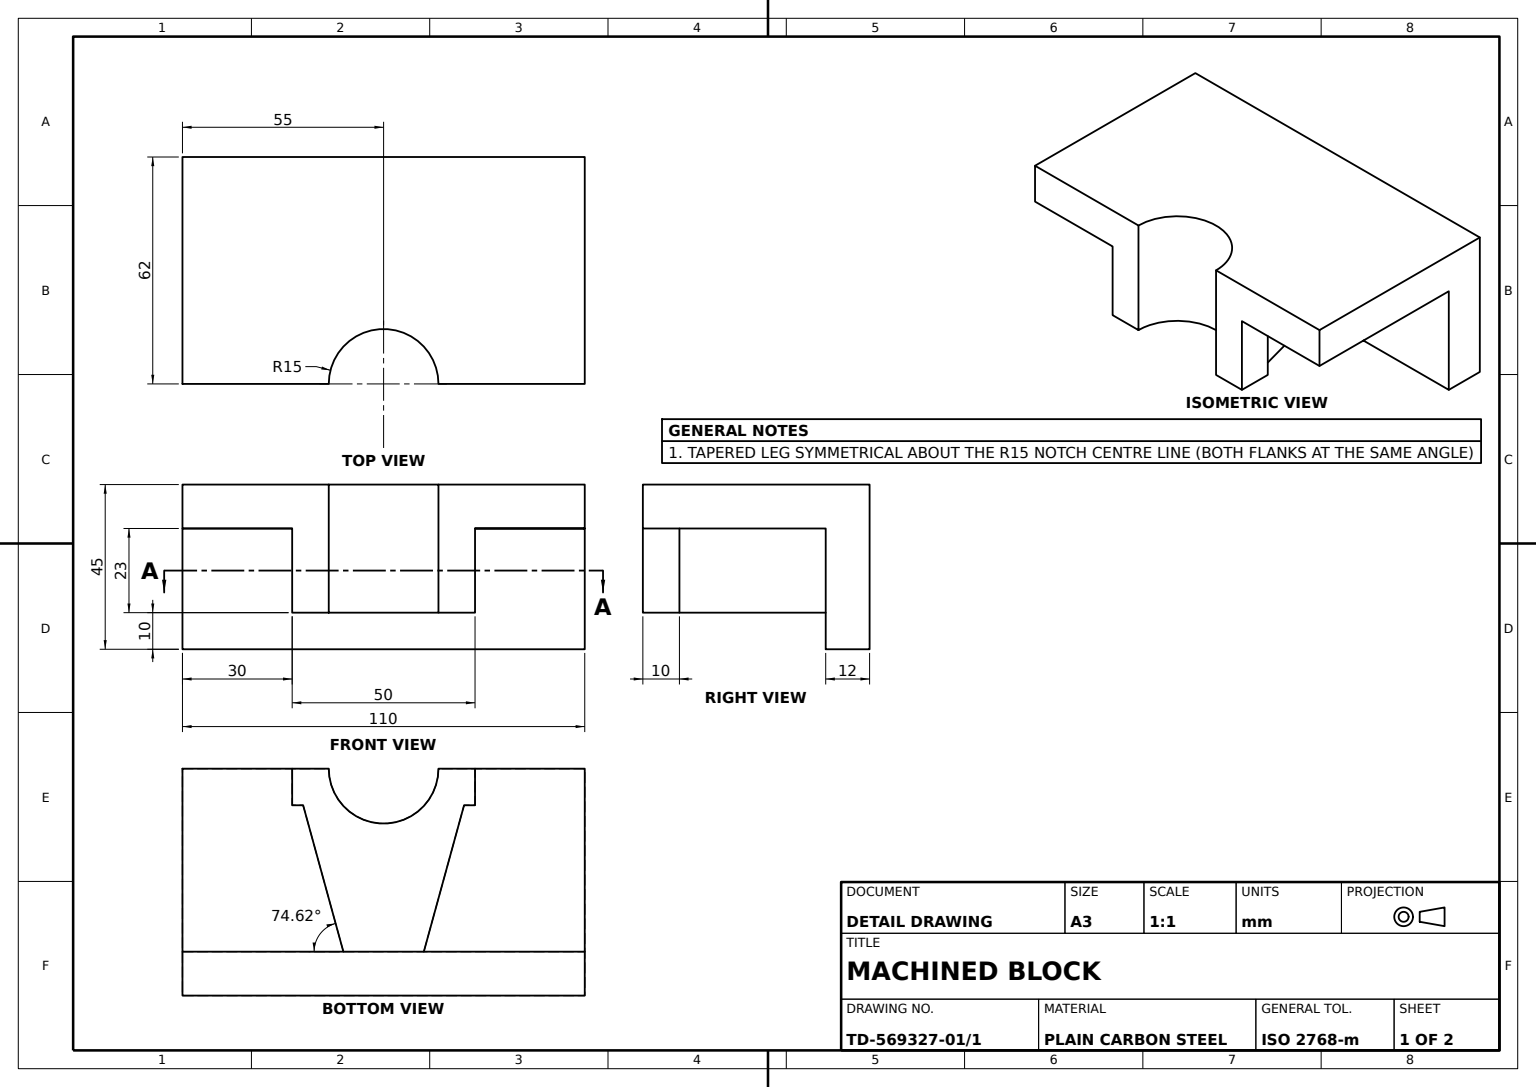
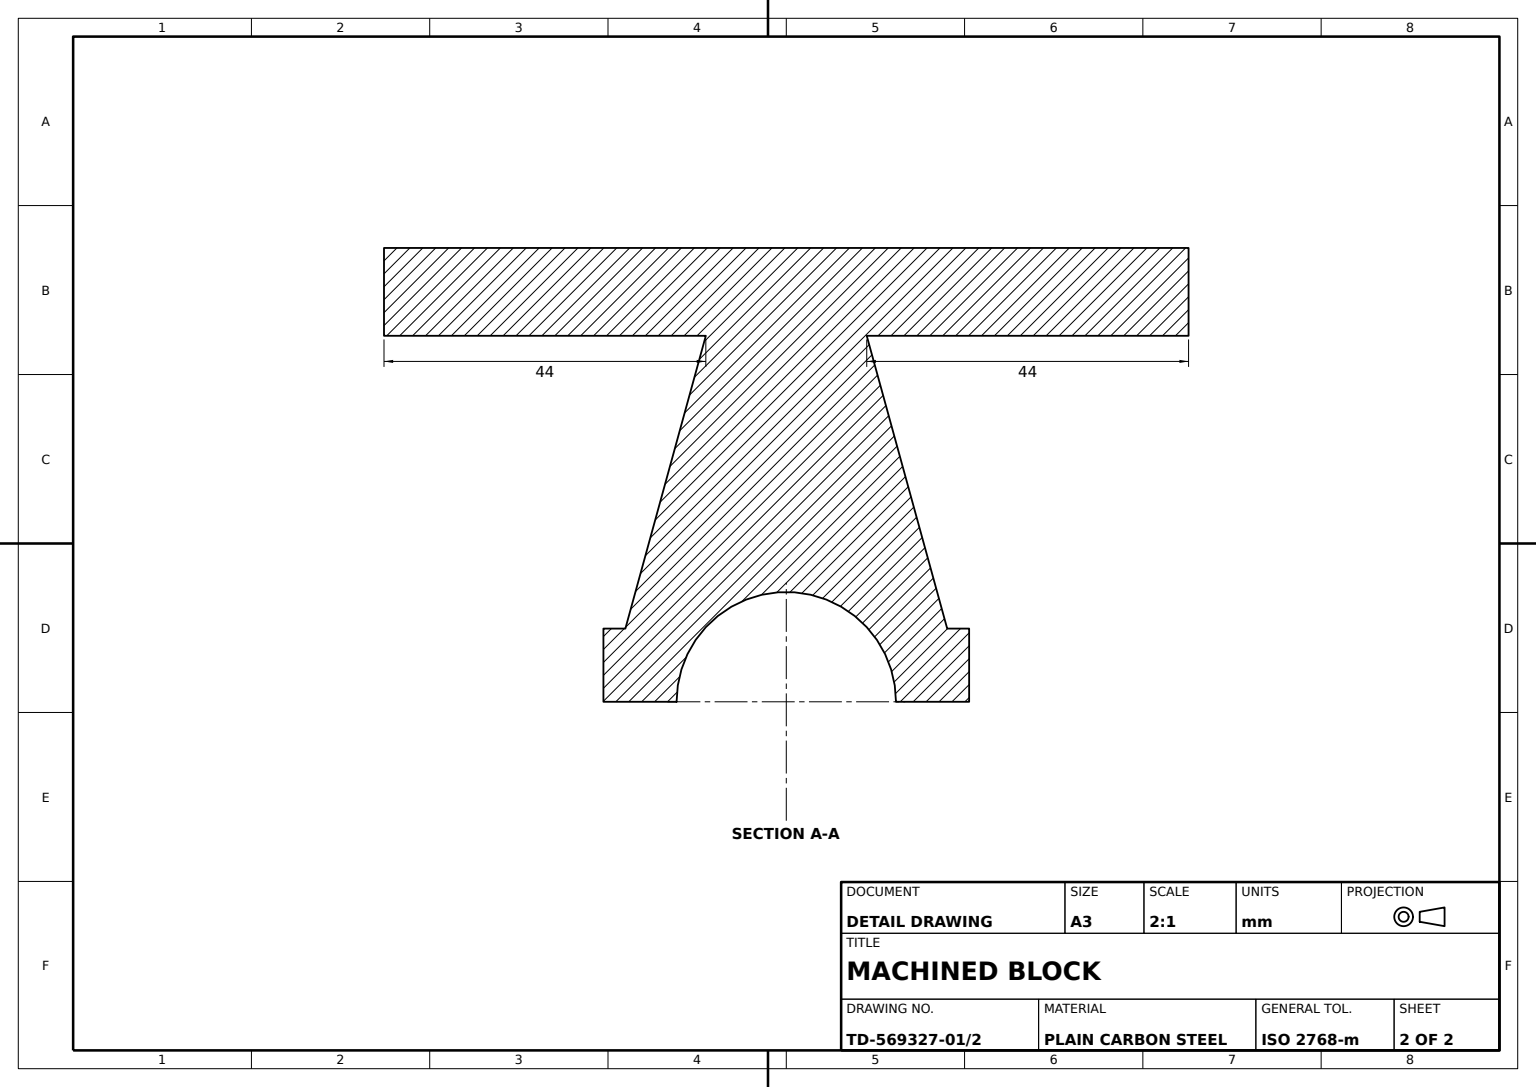
from build123d import *

# Parameters (mm, degrees)
BASE_PLATE_SKETCH_W          = 110
BASE_PLATE_SKETCH_H          = 45
BASE_PLATE_DEPTH             = 12
SECOND_BLOCK_SKETCH_W        = 110
SECOND_BLOCK_SKETCH_H        = 50
SECOND_BLOCK_DEPTH           = 12
LEG_PROFILE_BOSS_DEPTH       = 23
SEMICIRCULAR_START           = -12
SEMICIRCULAR_NOTCH_CUT_DEPTH = 12


with BuildPart() as part:
    # Base Plate Sketch → Base Plate (new body)
    with BuildSketch(Plane.XY):
        with Locations((55, 22.5)):
            Rectangle(BASE_PLATE_SKETCH_W, BASE_PLATE_SKETCH_H)
    extrude(amount=BASE_PLATE_DEPTH)

    # Second Block Sketch → Second Block (add)
    with BuildSketch(Plane(origin=(0, 45, 0), x_dir=(1, 0, 0), z_dir=(0, 1, 0))):
        with Locations((55, -37)):
            Rectangle(SECOND_BLOCK_SKETCH_W, SECOND_BLOCK_SKETCH_H)
    extrude(amount=-SECOND_BLOCK_DEPTH)

    # Leg Profile Sketch → Leg Profile Boss (add)
    with BuildSketch(Plane.XZ.offset(-33)):
        with BuildLine():
            Line((80, 62), (80, 52))
            Line((80, 52), (77, 52))
            Line((77, 52), (66, 12))
            Line((66, 12), (55, 12))
            Line((55, 12), (44, 12))
            Line((44, 12), (33, 52))
            Line((33, 52), (30, 52))
            Line((30, 52), (30, 62))
            Line((30, 62), (40, 62))
            ThreePointArc((40, 62), (55, 47), (70, 62))
            Line((70, 62), (80, 62))
        make_face()
    extrude(amount=LEG_PROFILE_BOSS_DEPTH)

    # Semicircular Notch Sketch → Semicircular Notch Cut (cut)
    with BuildSketch(Plane.XZ.offset(-33).offset(SEMICIRCULAR_START)):
        with BuildLine():
            Line((40, 62), (70, 62))
            ThreePointArc((70, 62), (55, 47), (40, 62))
        make_face()
    extrude(amount=SEMICIRCULAR_NOTCH_CUT_DEPTH, mode=Mode.SUBTRACT)


solid = part.part
